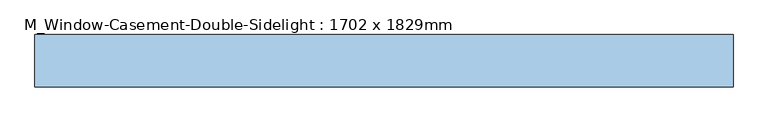
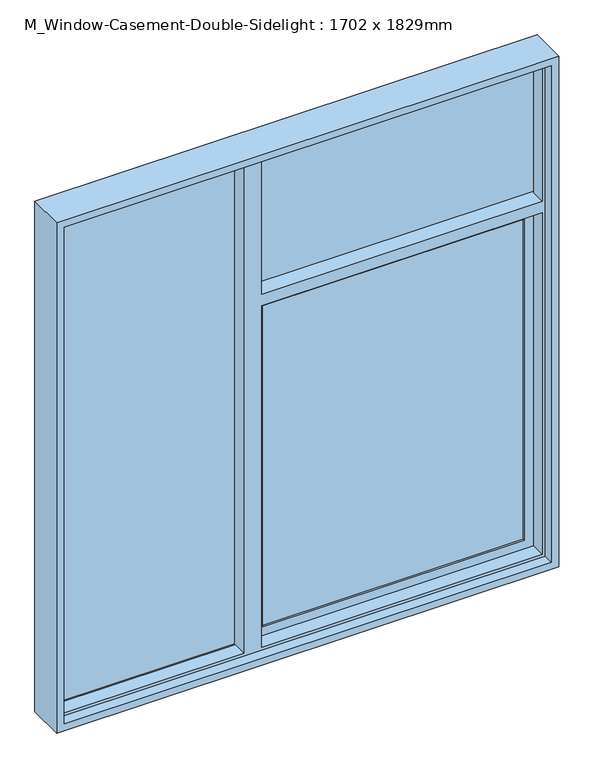
"""IFC4 building model written with IfcOpenShell, lengths in millimetres: window geometry, M_Window-Casement-Double-Sidelight : 1702 x 1829mm."""

from ifc_helpers import new_model, si_unit, frame, origin, place, context, project, spatial, polyline, outline, extrude, faceted_brep, source, transform, mapped, element, save


def m_window_casement_double_sidelight_1702_x_1829mm_92594323(model_context):
    return source(origin(), model_context, "Body", "SolidModel", [
        extrude(outline(polyline([(783.5796875, 47.6), (-102.8596875, 47.6), (-102.8596875, 60.3), (783.5796875, 60.3), (783.5796875, 47.6)])), frame((0.0, 0.0, 967.3203125), z_axis=(0.0, 0.0, 1.0), x_axis=(1.0, 0.0, 0.0)), (0.0, 0.0, 1.0), 1149.9592187),
        extrude(outline(polyline([(783.5796875, 34.9), (783.5796875, 28.55), (-102.8596875, 28.55), (-102.8596875, 34.9), (783.5796875, 34.9)])), frame((0.0, 0.0, 967.3203125), z_axis=(0.0, 0.0, 1.0), x_axis=(1.0, 0.0, 0.0)), (0.0, 0.0, 1.0), 1149.9592187),
        extrude(outline(polyline([(-195.58, 47.6), (-195.58, 41.25), (-825.5, 41.25), (-825.5, 47.6), (-195.58, 47.6)])), frame((0.0, 0.0, 935.5203125), z_axis=(0.0, 0.0, 1.0), x_axis=(1.0, 0.0, 0.0)), (0.0, 0.0, 1.0), 1767.8796875),
        extrude(outline(polyline([(-195.58, 34.9), (-195.58, 28.55), (-825.5, 28.55), (-825.5, 34.9), (-195.58, 34.9)])), frame((0.0, 0.0, 935.5203125), z_axis=(0.0, 0.0, 1.0), x_axis=(1.0, 0.0, 0.0)), (0.0, 0.0, 1.0), 1767.8796875),
        extrude(outline(polyline([(825.5, 34.9), (825.5, 28.55), (-144.78, 28.55), (-144.78, 34.9), (825.5, 34.9)])), frame((0.0, 0.0, 2201.1201563), z_axis=(0.0, 0.0, 1.0), x_axis=(1.0, 0.0, 0.0)), (0.0, 0.0, 1.0), 502.2798438),
        extrude(outline(polyline([(825.5, 47.6), (825.5, 41.25), (-144.78, 41.25), (-144.78, 47.6), (825.5, 47.6)])), frame((0.0, 0.0, 2201.1201563), z_axis=(0.0, 0.0, 1.0), x_axis=(1.0, 0.0, 0.0)), (0.0, 0.0, 1.0), 502.2798438),
        faceted_brep([(-825.5, 22.2, 2703.4), (-825.5, 63.5, 2703.4), (825.5, 63.5, 2703.4), (825.5, 22.2, 2703.4), (-144.78, 22.2, 2703.4), (-144.78, 60.3, 2703.4), (-195.58, 60.3, 2703.4), (-195.58, 22.2, 2703.4), (-815.3796875, -28.6, 2693.2796875), (-815.3796875, 22.2, 2693.2796875), (-195.58, 22.2, 2693.2796875), (-195.58, -28.6, 2693.2796875), (815.3796875, 22.2, 2693.2796875), (815.3796875, -28.6, 2693.2796875), (-134.6596875, -28.6, 2693.2796875), (-134.6596875, 22.2, 2693.2796875), (-825.5, -63.5, 2703.4), (-825.5, -28.6, 2703.4), (825.5, -28.6, 2703.4), (825.5, -63.5, 2703.4), (-850.9, 63.5, 2728.8), (-850.9, -63.5, 2728.8), (850.9, -63.5, 2728.8), (850.9, 63.5, 2728.8), (825.5, 63.5, 925.4), (825.5, 22.2, 925.4), (825.5, 22.2, 2159.1998438), (825.5, 60.3, 2159.1998438), (825.5, 60.3, 2201.1201563), (825.5, 22.2, 2201.1201563), (815.3796875, 22.2, 2201.1201563), (815.3796875, -28.6, 2201.1201563), (815.3796875, 22.2, 935.5203125), (815.3796875, -28.6, 935.5203125), (815.3796875, -28.6, 2159.1998438), (815.3796875, 22.2, 2159.1998438), (825.5, -28.6, 925.4), (825.5, -63.5, 925.4), (850.9, -63.5, 900.0), (850.9, 63.5, 900.0), (-825.5, 63.5, 925.4), (-825.5, 22.2, 925.4), (-195.58, 22.2, 925.4), (-195.58, 60.3, 925.4), (-144.78, 60.3, 925.4), (-144.78, 22.2, 925.4), (-134.6596875, 22.2, 935.5203125), (-134.6596875, -28.6, 935.5203125), (-815.3796875, 22.2, 935.5203125), (-815.3796875, -28.6, 935.5203125), (-195.58, -28.6, 935.5203125), (-195.58, 22.2, 935.5203125), (-825.5, -28.6, 925.4), (-825.5, -63.5, 925.4), (-850.9, -63.5, 900.0), (-850.9, 63.5, 900.0), (-134.6596875, 22.2, 2201.1201563), (-144.78, 22.2, 2201.1201563), (-144.78, 22.2, 2159.1998438), (-134.6596875, 22.2, 2159.1998438), (-134.6596875, -28.6, 2201.1201563), (-134.6596875, -28.6, 2159.1998438), (-144.78, 60.3, 2201.1201563), (-144.78, 60.3, 2159.1998438)], [[[0, 1, 2, 3, 4, 5, 6, 7]], [[8, 9, 10, 11]], [[12, 13, 14, 15]], [[16, 17, 18, 19]], [[20, 21, 22, 23]], [[3, 2, 24, 25, 26, 27, 28, 29]], [[13, 12, 30, 31]], [[32, 33, 34, 35]], [[19, 18, 36, 37]], [[23, 22, 38, 39]], [[25, 24, 40, 41, 42, 43, 44, 45]], [[33, 32, 46, 47]], [[48, 49, 50, 51]], [[37, 36, 52, 53]], [[39, 38, 54, 55]], [[1, 0, 41, 40]], [[12, 15, 56, 57, 4, 3, 29, 30]], [[46, 32, 35, 26, 25, 45, 58, 59]], [[41, 0, 7, 10, 9, 48, 51, 42]], [[9, 8, 49, 48]], [[17, 52, 36, 18], [13, 31, 60, 14], [33, 47, 61, 34], [49, 8, 11, 50]], [[17, 16, 53, 52]], [[22, 21, 54, 38], [16, 19, 37, 53]], [[21, 20, 55, 54]], [[20, 23, 39, 55], [2, 1, 40, 24]], [[43, 6, 5, 62, 28, 27, 63, 44]], [[6, 43, 42, 51, 50, 11, 10, 7]], [[15, 14, 60, 56]], [[47, 46, 59, 61]], [[5, 4, 57, 62]], [[45, 44, 63, 58]], [[63, 27, 26, 35, 34, 61, 59, 58]], [[28, 62, 57, 56, 60, 31, 30, 29]]]),
        extrude(outline(polyline([(2159.1998438, 825.5), (2159.1998438, -144.78), (925.4, -144.78), (925.4, 825.5), (2159.1998438, 825.5)]), holes=[polyline([(967.3203125, 783.5796875), (967.3203125, -102.8596875), (2117.2795313, -102.8596875), (2117.2795313, 783.5796875), (967.3203125, 783.5796875)])]), frame((0.0, 22.2, 0.0), z_axis=(0.0, 1.0, 0.0), x_axis=(0.0, 0.0, 1.0)), (0.0, 0.0, 1.0), 31.75),
    ])


if __name__ == "__main__":
    model = new_model("IFC4")
    model_context = context("Model", 3, world=origin())
    ifc_project = project(units=[si_unit("LENGTHUNIT", "METRE", prefix="MILLI")], contexts=[model_context])
    site = spatial("IfcSite", under=ifc_project)
    building = spatial("IfcBuilding", under=site)
    placement = place(None, origin())
    m_window_casement_double_sidelight_1702_x_1829mm_shape = m_window_casement_double_sidelight_1702_x_1829mm_92594323(model_context)
    element("IfcWindow", 1, ObjectType="M_Window-Casement-Double-Sidelight : 1702 x 1829mm", at=placement, inside=building, context=model_context, shape_type="MappedRepresentation", body=[
        mapped(m_window_casement_double_sidelight_1702_x_1829mm_shape, transform((0.0, 0.0, 0.0), x_axis=(1.0, 0.0, 0.0), y_axis=(0.0, 1.0, 0.0), z_axis=(0.0, 0.0, 1.0))),
    ])
    save(model, "model.ifc")

# Revit data of these elements
# Type "M_Window-Casement-Double-Sidelight : 1702 x 1829mm"
#   Type Mark = "18"
#   Fire Rating = "0.5h"
#   Assembly Code = "B2020100"
#   Analytic Construction = "Double glazing - domestic"
#   Window Inset [instance default] = 0' - 0.62598"
#   Wall Thickness [instance default] = 0' - 5.90551"
#   Visual Light Transmittance = 0.81
#   Transom Height Ratio = 0.3
#   Transom Height = 1' - 9.6"
#   Thermal Resistance (R) = 1.8146 (h·ft²·°F)/BTU
#   Solar Heat Gain Coefficient = 0.76
#   Side Width = 2' - 2.8"
#   Rough Width = 5' - 7.59055"
#   Rough Height = 6' - 0.59055"
#   Opening Window Width = 3' - 4.2"
#   Opening Window Height = 4' - 2.4"
#   Heat Transfer Coefficient (U) = 0.5511 BTU/(h·ft²·°F)
#   Height = 6' - 0"
#   Frame Gap 3 [instance default] = 0' - 1.65041"
#   Frame Gap 2 [instance default] = 0' - 0.62598"
#   Frame Gap 1 = 0' - 1 51/128"
#   Default Sill Height = 2' - 11.43307"
#   Width = 5' - 7"
#   Frame Material = Metal - Aluminum
#   Glass Panel Material = Glass
#   Wall Closure = (empty or 0)
# Element 1 (IfcWindow, "M_Window-Casement-Double-Sidelight : 1702 x 1829mm")
#   Wall Thickness = 0' - 5"
#   Materials on its faces: "Metal - Aluminum", "Glass"
# Materials
#   "Metal - Aluminum": class "Metal", colour RGB 247 247 247, transparency 0
#   "Glass": class "Glass", colour RGB 0 128 192, transparency 0.75, Description = "Soda Lime Glass", Cost = 0
